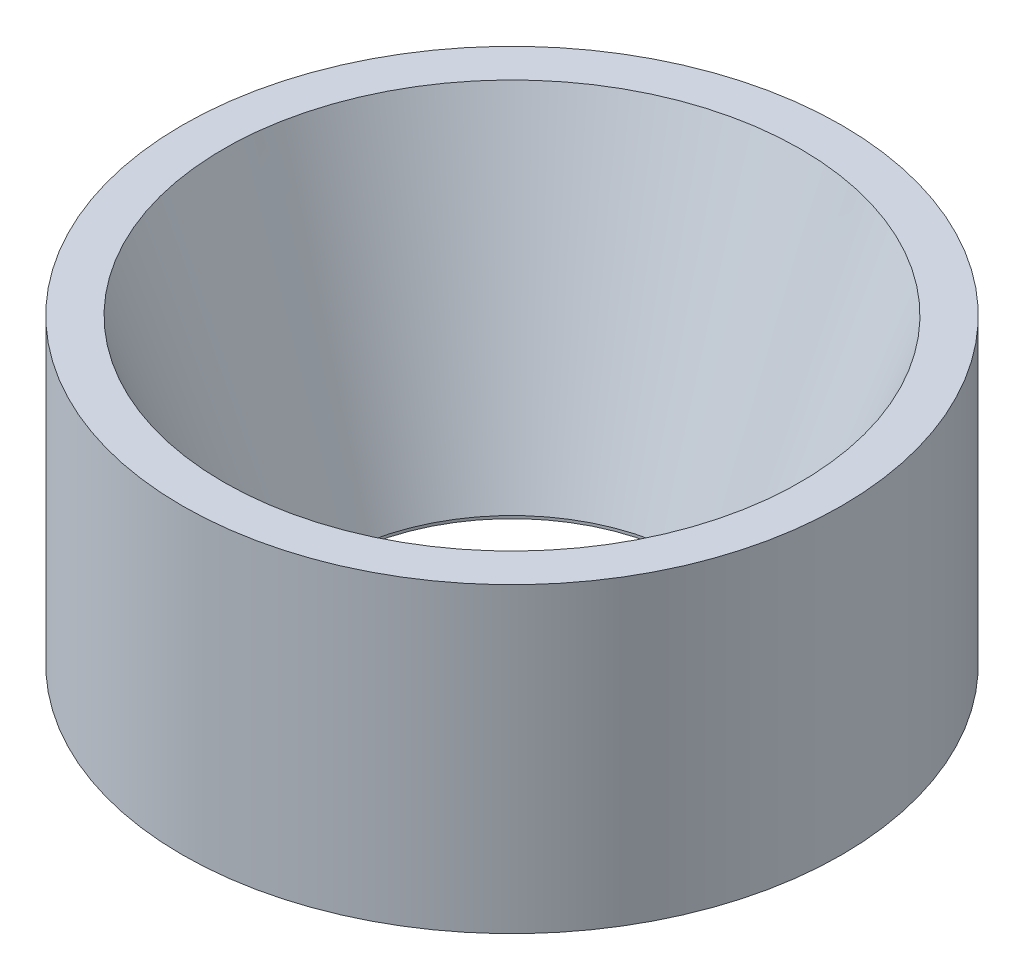
SolidWorks part; units mm, degrees
material "Plain Carbon Steel"
ref_plane "Front Plane" through (0, 0, 0) normal (0, 0, 1) x (1, 0, 0)
ref_plane "Top Plane" through (0, 0, 0) normal (0, 1, 0) x (1, 0, 0)
ref_plane "Right Plane" through (0, 0, 0) normal (1, 0, 0) x (0, 0, -1)
sketch "Ring Outline Sketch Ø48" plane through (0, 0, 0) normal (0, 1, 0) x (1, 0, 0)
  line L0 (0, 40.1129) -> (0, -45.5289) construction
  line L1 (76.615, 0) -> (-58.3357, 0) construction
  circle A0 centre (0, 0) radius 24
  dimension "D1" = 48
extrude "Ring Body Ø48x22" add sketch "Ring Outline Sketch Ø48" along normal blind 22
sketch "Taper Top Profile Ø40" plane through (0, 22, 0) normal (0, 1, 0) x (1, 0, 0)
  circle A0 centre (0, 0) radius 21
  dimension "D1" = 42
ref_plane "Taper Bottom Plane 16mm" through (0, 0.2, 0) normal (0, 1, 0) x (1, 0, 0)
sketch "Taper Bottom Profile Ø20" plane through (0, 0.2, 0) normal (0, 1, 0) x (1, 0, 0)
  circle A0 centre (0, 0) radius 13
  dimension "D1" = 26
loft "Conical Bore Ø40-Ø20" cut profiles "Taper Top Profile Ø40", "Taper Bottom Profile Ø20"
sketch "Through Bore Sketch Ø20" plane through (0, 0.2, 0) normal (0, 1, 0) x (1, 0, 0)
  circle A0 centre (0, 0) radius 13
  dimension "D1" = 26
extrude "Through Bore Ø20" cut sketch "Through Bore Sketch Ø20" against normal up to next
